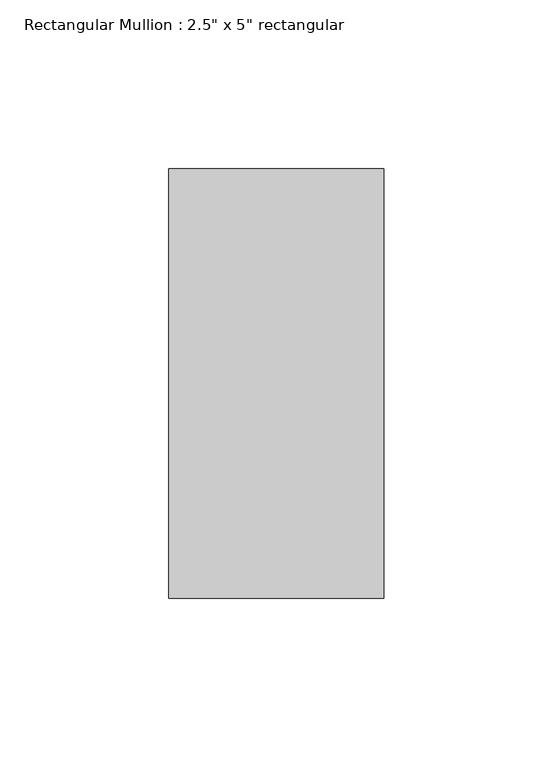
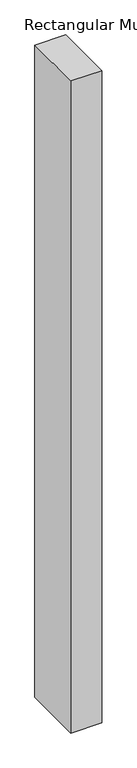
"""IFC4 building model written with IfcOpenShell, lengths in millimetres: member geometry."""

from ifc_helpers import new_model, si_unit, frame, origin, place, context, project, spatial, polyline, outline, extrude, source, transform, mapped, element, save


def member_e1556d54(model_context):
    return source(origin(), model_context, "Body", "SweptSolid", [
        extrude(outline(polyline([(0.0, 63.5), (0.0, -63.5), (-63.5, -63.5), (-63.5, 63.5), (0.0, 63.5)])), frame((0.0, 0.0, -1410.3945466), z_axis=(0.0, 0.0, 1.0), x_axis=(1.0, 0.0, 0.0)), (0.0, 0.0, 1.0), 1410.3945466),
    ])


if __name__ == "__main__":
    model = new_model("IFC4")
    model_context = context("Model", 3, world=origin())
    ifc_project = project(units=[si_unit("LENGTHUNIT", "METRE", prefix="MILLI")], contexts=[model_context])
    site = spatial("IfcSite", under=ifc_project)
    building = spatial("IfcBuilding", under=site)
    placement = place(None, origin())
    member_shape = member_e1556d54(model_context)
    element("IfcMember", 1, ObjectType="Rectangular Mullion : 2.5\" x 5\" rectangular", at=placement, inside=building, context=model_context, shape_type="MappedRepresentation", body=[
        mapped(member_shape, transform((0.0, 0.0, 0.0), x_axis=(1.0, 0.0, 0.0), y_axis=(0.0, 1.0, 0.0), z_axis=(0.0, 0.0, 1.0))),
    ])
    save(model, "model.ifc")

# Revit data of these elements
# Type "Rectangular Mullion : 2.5\" x 5\" rectangular"
#   built-in parameter 1007304 = 0.416667 (stored number, unit not read)
#   built-in parameter 1007301 = 0.104167 (stored number, unit not read)
#   built-in parameter 1007300 = 0.104167 (stored number, unit not read)
# Element 1 (IfcMember, "Rectangular Mullion : 2.5\" x 5\" rectangular")
#   Materials on its faces: "Aluminum"
# Materials
#   "Aluminum": class "Metal", colour RGB 247 247 247, transparency 0, Description = "Aluminum 6061", Cost = 0
